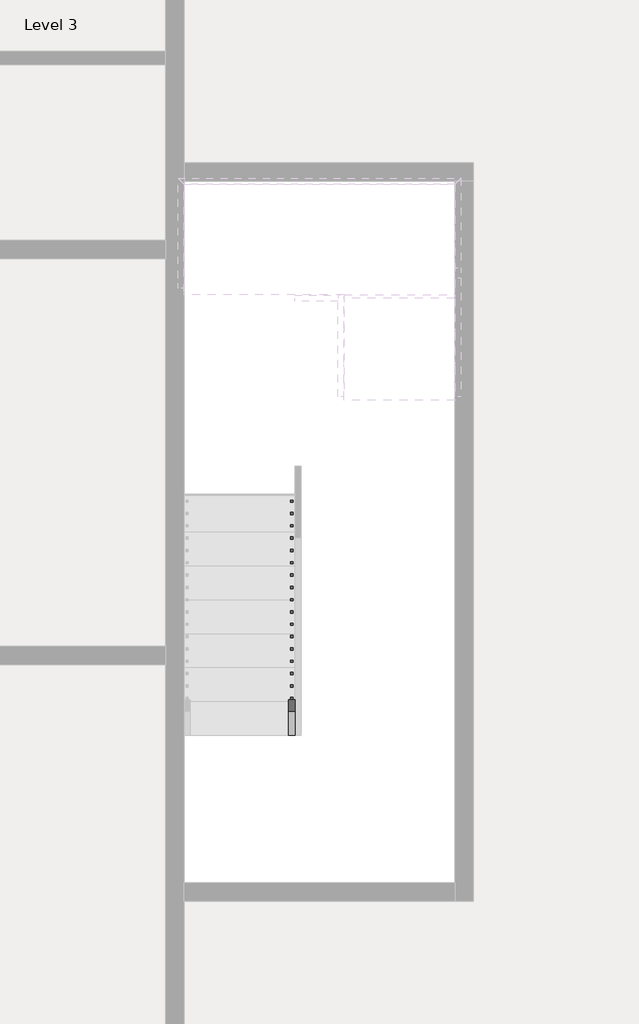
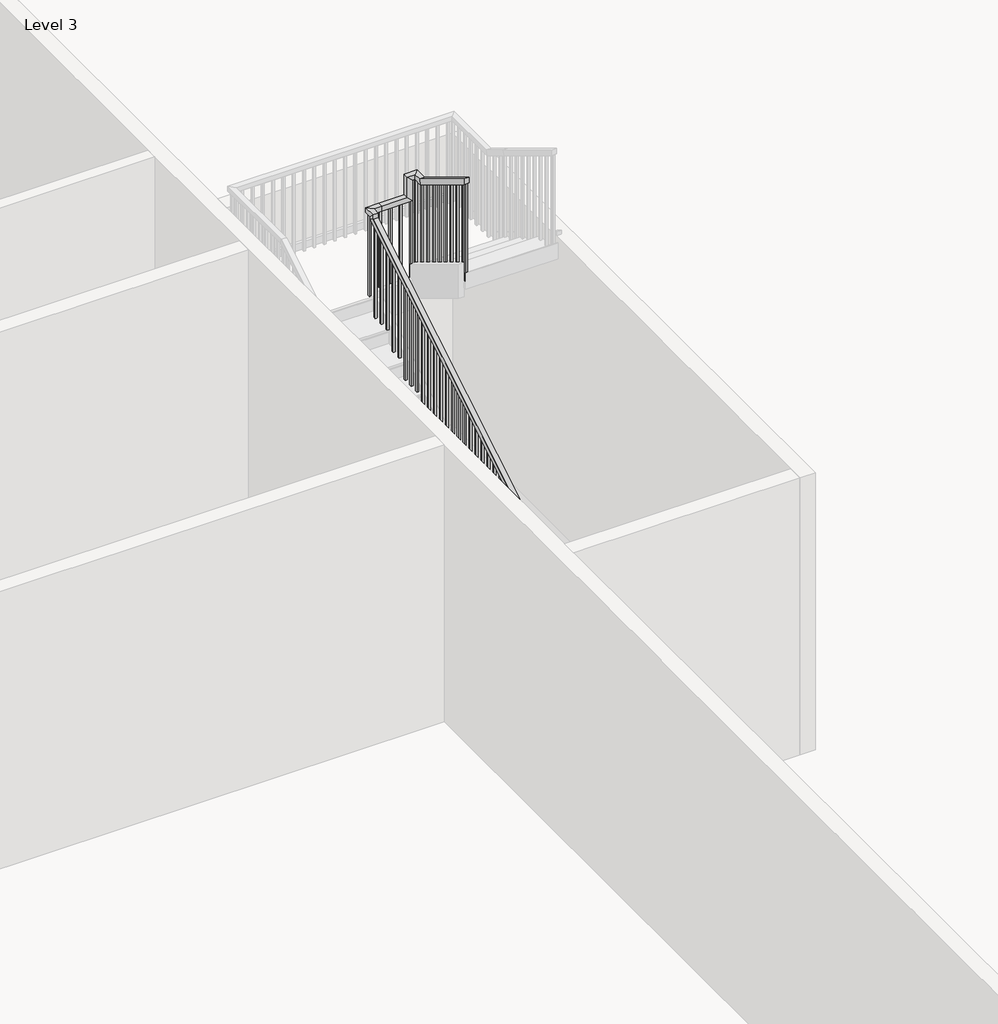
# One storey, part 5 of 8: 1 railing.
"""IFC4 building model written with IfcOpenShell, lengths in millimetres."""

from ifc_helpers import new_model, si_unit, frame, origin, place, context, project, spatial, polyline, outline, extrude, faceted_brep, element, save

model = new_model("IFC4")

# Units and contexts
model_context = context("Model", 3, world=origin())
ifc_project = project(units=[si_unit("LENGTHUNIT", "METRE", prefix="MILLI")], contexts=[model_context])

# Site, building, storey
site = spatial("IfcSite", under=ifc_project)
building = spatial("IfcBuilding", under=site)
storey = spatial("IfcBuildingStorey", under=building, Name="Level 3", Elevation=31330.6172466)

# Railing
placement = place(None, origin())
element("IfcRailing", 1, ObjectType="Handrail - Rectangular", at=placement, inside=storey, context=model_context, shape_type="SolidModel", body=[
    faceted_brep([(-2753.8415084, -23154.3851539, 32414.3505799), (-2753.8415084, -23154.3851539, 32354.9491197), (-2703.0415084, -23154.3851539, 32354.9491197), (-2703.0415084, -23154.3851539, 32414.3505799), (-2753.8415084, -19598.3851539, 34569.5020951), (-2753.8415084, -19547.5851539, 34540.8885136), (-2703.0415084, -19547.5851539, 34540.8885136), (-2703.0415084, -19598.3851539, 34569.5020951), (-2753.8415084, -19598.3851539, 34615.6839133), (-2753.8415084, -19547.5851539, 34564.8839133), (-2703.0415084, -19547.5851539, 34564.8839133), (-2703.0415084, -19598.3851539, 34615.6839133), (-2753.8415084, -19471.3851539, 34615.6839133), (-2753.8415084, -19471.3851539, 34564.8839133), (-2703.0415084, -19522.1851539, 34564.8839133), (-2703.0415084, -19522.1851539, 34615.6839133), (-2626.8415084, -19471.3851539, 34615.6839133), (-2626.8415084, -19471.3851539, 34564.8839133), (-2626.8415084, -19522.1851539, 34564.8839133), (-2626.8415084, -19522.1851539, 34615.6839133), (-2372.8415084, -19471.3851539, 34615.6839133), (-2322.0415084, -19471.3851539, 34564.8839133), (-2322.0415084, -19522.1851539, 34564.8839133), (-2372.8415084, -19522.1851539, 34615.6839133), (-2372.8415084, -19471.3851539, 34831.1990648), (-2322.0415084, -19471.3851539, 34780.3990648), (-2322.0415084, -19522.1851539, 34780.3990648), (-2372.8415084, -19522.1851539, 34831.1990648), (-2245.8415084, -19471.3851539, 34831.1990648), (-2245.8415084, -19471.3851539, 34780.3990648), (-2296.6415084, -19522.1851539, 34780.3990648), (-2296.6415084, -19522.1851539, 34831.1990648), (-2245.8415084, -19598.3851539, 34831.1990648), (-2245.8415084, -19612.5775633, 34780.3990648), (-2296.6415084, -19612.5775633, 34780.3990648), (-2296.6415084, -19598.3851539, 34831.1990648), (-2245.8415084, -20360.3851539, 35293.0172466), (-2296.6415084, -20360.3851539, 35293.0172466), (-2296.6415084, -20360.3851539, 35233.6157863), (-2245.8415084, -20360.3851539, 35233.6157863)], [[[0, 1, 2, 3]], [[1, 0, 4, 5]], [[2, 1, 5, 6]], [[3, 2, 6, 7]], [[0, 3, 7, 4]], [[5, 4, 8, 9]], [[6, 5, 9, 10]], [[7, 6, 10, 11]], [[4, 7, 11, 8]], [[9, 8, 12, 13]], [[10, 9, 13, 14]], [[11, 10, 14, 15]], [[8, 11, 15, 12]], [[13, 12, 16, 17]], [[14, 13, 17, 18]], [[15, 14, 18, 19]], [[12, 15, 19, 16]], [[17, 16, 20, 21]], [[18, 17, 21, 22]], [[19, 18, 22, 23]], [[16, 19, 23, 20]], [[21, 20, 24, 25]], [[22, 21, 25, 26]], [[23, 22, 26, 27]], [[20, 23, 27, 24]], [[25, 24, 28, 29]], [[26, 25, 29, 30]], [[27, 26, 30, 31]], [[24, 27, 31, 28]], [[29, 28, 32, 33]], [[30, 29, 33, 34]], [[31, 30, 34, 35]], [[28, 31, 35, 32]], [[36, 37, 38, 39]], [[33, 32, 36, 39]], [[34, 33, 39, 38]], [[35, 34, 38, 37]], [[32, 35, 37, 36]]]),
    extrude(outline(polyline([(-20319.1101539, 35208.6006348), (-20300.0601539, 35197.0551803), (-20300.0601539, 34209.2839133), (-20319.1101539, 34209.2839133), (-20319.1101539, 35208.6006348)])), frame((-2280.7665084, 0.0, 0.0), z_axis=(1.0, 0.0, 0.0), x_axis=(0.0, 1.0, 0.0)), (0.0, 0.0, 1.0), 19.05),
    extrude(outline(polyline([(-20217.5101539, 35147.0248773), (-20198.4601539, 35135.4794227), (-20198.4601539, 34209.2839133), (-20217.5101539, 34209.2839133), (-20217.5101539, 35147.0248773)])), frame((-2280.7665084, 0.0, 0.0), z_axis=(1.0, 0.0, 0.0), x_axis=(0.0, 1.0, 0.0)), (0.0, 0.0, 1.0), 19.05),
    extrude(outline(polyline([(-20115.9101539, 35085.4491197), (-20096.8601539, 35073.9036651), (-20096.8601539, 34209.2839133), (-20115.9101539, 34209.2839133), (-20115.9101539, 35085.4491197)])), frame((-2280.7665084, 0.0, 0.0), z_axis=(1.0, 0.0, 0.0), x_axis=(0.0, 1.0, 0.0)), (0.0, 0.0, 1.0), 19.05),
    extrude(outline(polyline([(-20014.3101539, 35023.8733621), (-19995.2601539, 35012.3279076), (-19995.2601539, 34039.9505799), (-20014.3101539, 34039.9505799), (-20014.3101539, 35023.8733621)])), frame((-2280.7665084, 0.0, 0.0), z_axis=(1.0, 0.0, 0.0), x_axis=(0.0, 1.0, 0.0)), (0.0, 0.0, 1.0), 19.05),
    extrude(outline(polyline([(-19912.7101539, 34962.2976045), (-19893.6601539, 34950.75215), (-19893.6601539, 34039.9505799), (-19912.7101539, 34039.9505799), (-19912.7101539, 34962.2976045)])), frame((-2280.7665084, 0.0, 0.0), z_axis=(1.0, 0.0, 0.0), x_axis=(0.0, 1.0, 0.0)), (0.0, 0.0, 1.0), 19.05),
    extrude(outline(polyline([(-19811.1101539, 34900.721847), (-19792.0601539, 34889.1763924), (-19792.0601539, 34039.9505799), (-19811.1101539, 34039.9505799), (-19811.1101539, 34900.721847)])), frame((-2280.7665084, 0.0, 0.0), z_axis=(1.0, 0.0, 0.0), x_axis=(0.0, 1.0, 0.0)), (0.0, 0.0, 1.0), 19.05),
    extrude(outline(polyline([(-19709.5101539, 34839.1460894), (-19690.4601539, 34827.6006348), (-19690.4601539, 33870.6172466), (-19709.5101539, 33870.6172466), (-19709.5101539, 34839.1460894)])), frame((-2280.7665084, 0.0, 0.0), z_axis=(1.0, 0.0, 0.0), x_axis=(0.0, 1.0, 0.0)), (0.0, 0.0, 1.0), 19.05),
    extrude(outline(polyline([(-19607.9101539, 34777.5703318), (-19588.8601539, 34766.0248773), (-19588.8601539, 33870.6172466), (-19607.9101539, 33870.6172466), (-19607.9101539, 34777.5703318)])), frame((-2280.7665084, 0.0, 0.0), z_axis=(1.0, 0.0, 0.0), x_axis=(0.0, 1.0, 0.0)), (0.0, 0.0, 1.0), 19.05),
    extrude(outline(polyline([(-2331.5665084, -19506.3101539), (-2331.5665084, -19487.2601539), (-2312.5165084, -19487.2601539), (-2312.5165084, -19506.3101539), (-2331.5665084, -19506.3101539)])), frame((0.0, 0.0, 33701.2839133), z_axis=(0.0, 0.0, 1.0), x_axis=(1.0, 0.0, 0.0)), (0.0, 0.0, 1.0), 1079.1151515),
    extrude(outline(polyline([(-2433.1665084, -19506.3101539), (-2433.1665084, -19487.2601539), (-2414.1165084, -19487.2601539), (-2414.1165084, -19506.3101539), (-2433.1665084, -19506.3101539)])), frame((0.0, 0.0, 33701.2839133), z_axis=(0.0, 0.0, 1.0), x_axis=(1.0, 0.0, 0.0)), (0.0, 0.0, 1.0), 863.6),
    extrude(outline(polyline([(-2534.7665084, -19506.3101539), (-2534.7665084, -19487.2601539), (-2515.7165084, -19487.2601539), (-2515.7165084, -19506.3101539), (-2534.7665084, -19506.3101539)])), frame((0.0, 0.0, 33701.2839133), z_axis=(0.0, 0.0, 1.0), x_axis=(1.0, 0.0, 0.0)), (0.0, 0.0, 1.0), 863.6),
    extrude(outline(polyline([(-2636.3665084, -19506.3101539), (-2636.3665084, -19487.2601539), (-2617.3165084, -19487.2601539), (-2617.3165084, -19506.3101539), (-2636.3665084, -19506.3101539)])), frame((0.0, 0.0, 33701.2839133), z_axis=(0.0, 0.0, 1.0), x_axis=(1.0, 0.0, 0.0)), (0.0, 0.0, 1.0), 863.6),
    extrude(outline(polyline([(-19607.9101539, 34504.3279076), (-19588.8601539, 34515.8733621), (-19588.8601539, 33531.9505799), (-19607.9101539, 33531.9505799), (-19607.9101539, 34504.3279076)])), frame((-2737.9665084, 0.0, 0.0), z_axis=(1.0, 0.0, 0.0), x_axis=(0.0, 1.0, 0.0)), (0.0, 0.0, 1.0), 19.05),
    extrude(outline(polyline([(-19709.5101539, 34442.75215), (-19690.4601539, 34454.2976045), (-19690.4601539, 33531.9505799), (-19709.5101539, 33531.9505799), (-19709.5101539, 34442.75215)])), frame((-2737.9665084, 0.0, 0.0), z_axis=(1.0, 0.0, 0.0), x_axis=(0.0, 1.0, 0.0)), (0.0, 0.0, 1.0), 19.05),
    extrude(outline(polyline([(-19811.1101539, 34381.1763924), (-19792.0601539, 34392.721847), (-19792.0601539, 33531.9505799), (-19811.1101539, 33531.9505799), (-19811.1101539, 34381.1763924)])), frame((-2737.9665084, 0.0, 0.0), z_axis=(1.0, 0.0, 0.0), x_axis=(0.0, 1.0, 0.0)), (0.0, 0.0, 1.0), 19.05),
    extrude(outline(polyline([(-19912.7101539, 34319.6006348), (-19893.6601539, 34331.1460894), (-19893.6601539, 33362.6172466), (-19912.7101539, 33362.6172466), (-19912.7101539, 34319.6006348)])), frame((-2737.9665084, 0.0, 0.0), z_axis=(1.0, 0.0, 0.0), x_axis=(0.0, 1.0, 0.0)), (0.0, 0.0, 1.0), 19.05),
    extrude(outline(polyline([(-20014.3101539, 34258.0248773), (-19995.2601539, 34269.5703318), (-19995.2601539, 33362.6172466), (-20014.3101539, 33362.6172466), (-20014.3101539, 34258.0248773)])), frame((-2737.9665084, 0.0, 0.0), z_axis=(1.0, 0.0, 0.0), x_axis=(0.0, 1.0, 0.0)), (0.0, 0.0, 1.0), 19.05),
    extrude(outline(polyline([(-20115.9101539, 34196.4491197), (-20096.8601539, 34207.9945742), (-20096.8601539, 33193.2839133), (-20115.9101539, 33193.2839133), (-20115.9101539, 34196.4491197)])), frame((-2737.9665084, 0.0, 0.0), z_axis=(1.0, 0.0, 0.0), x_axis=(0.0, 1.0, 0.0)), (0.0, 0.0, 1.0), 19.05),
    extrude(outline(polyline([(-20217.5101539, 34134.8733621), (-20198.4601539, 34146.4188166), (-20198.4601539, 33193.2839133), (-20217.5101539, 33193.2839133), (-20217.5101539, 34134.8733621)])), frame((-2737.9665084, 0.0, 0.0), z_axis=(1.0, 0.0, 0.0), x_axis=(0.0, 1.0, 0.0)), (0.0, 0.0, 1.0), 19.05),
    extrude(outline(polyline([(-20319.1101539, 34073.2976045), (-20300.0601539, 34084.8430591), (-20300.0601539, 33193.2839133), (-20319.1101539, 33193.2839133), (-20319.1101539, 34073.2976045)])), frame((-2737.9665084, 0.0, 0.0), z_axis=(1.0, 0.0, 0.0), x_axis=(0.0, 1.0, 0.0)), (0.0, 0.0, 1.0), 19.05),
    extrude(outline(polyline([(-20420.7101539, 34011.721847), (-20401.6601539, 34023.2673015), (-20401.6601539, 33023.9505799), (-20420.7101539, 33023.9505799), (-20420.7101539, 34011.721847)])), frame((-2737.9665084, 0.0, 0.0), z_axis=(1.0, 0.0, 0.0), x_axis=(0.0, 1.0, 0.0)), (0.0, 0.0, 1.0), 19.05),
    extrude(outline(polyline([(-20522.3101539, 33950.1460894), (-20503.2601539, 33961.6915439), (-20503.2601539, 33023.9505799), (-20522.3101539, 33023.9505799), (-20522.3101539, 33950.1460894)])), frame((-2737.9665084, 0.0, 0.0), z_axis=(1.0, 0.0, 0.0), x_axis=(0.0, 1.0, 0.0)), (0.0, 0.0, 1.0), 19.05),
    extrude(outline(polyline([(-20623.9101539, 33888.5703318), (-20604.8601539, 33900.1157863), (-20604.8601539, 33023.9505799), (-20623.9101539, 33023.9505799), (-20623.9101539, 33888.5703318)])), frame((-2737.9665084, 0.0, 0.0), z_axis=(1.0, 0.0, 0.0), x_axis=(0.0, 1.0, 0.0)), (0.0, 0.0, 1.0), 19.05),
    extrude(outline(polyline([(-20725.5101539, 33826.9945742), (-20706.4601539, 33838.5400288), (-20706.4601539, 32854.6172466), (-20725.5101539, 32854.6172466), (-20725.5101539, 33826.9945742)])), frame((-2737.9665084, 0.0, 0.0), z_axis=(1.0, 0.0, 0.0), x_axis=(0.0, 1.0, 0.0)), (0.0, 0.0, 1.0), 19.05),
    extrude(outline(polyline([(-20827.1101539, 33765.4188166), (-20808.0601539, 33776.9642712), (-20808.0601539, 32854.6172466), (-20827.1101539, 32854.6172466), (-20827.1101539, 33765.4188166)])), frame((-2737.9665084, 0.0, 0.0), z_axis=(1.0, 0.0, 0.0), x_axis=(0.0, 1.0, 0.0)), (0.0, 0.0, 1.0), 19.05),
    extrude(outline(polyline([(-20928.7101539, 33703.8430591), (-20909.6601539, 33715.3885136), (-20909.6601539, 32854.6172466), (-20928.7101539, 32854.6172466), (-20928.7101539, 33703.8430591)])), frame((-2737.9665084, 0.0, 0.0), z_axis=(1.0, 0.0, 0.0), x_axis=(0.0, 1.0, 0.0)), (0.0, 0.0, 1.0), 19.05),
    extrude(outline(polyline([(-21030.3101539, 33642.2673015), (-21011.2601539, 33653.812756), (-21011.2601539, 32685.2839133), (-21030.3101539, 32685.2839133), (-21030.3101539, 33642.2673015)])), frame((-2737.9665084, 0.0, 0.0), z_axis=(1.0, 0.0, 0.0), x_axis=(0.0, 1.0, 0.0)), (0.0, 0.0, 1.0), 19.05),
    extrude(outline(polyline([(-21131.9101539, 33580.6915439), (-21112.8601539, 33592.2369985), (-21112.8601539, 32685.2839133), (-21131.9101539, 32685.2839133), (-21131.9101539, 33580.6915439)])), frame((-2737.9665084, 0.0, 0.0), z_axis=(1.0, 0.0, 0.0), x_axis=(0.0, 1.0, 0.0)), (0.0, 0.0, 1.0), 19.05),
    extrude(outline(polyline([(-21233.5101539, 33519.1157863), (-21214.4601539, 33530.6612409), (-21214.4601539, 32515.9505799), (-21233.5101539, 32515.9505799), (-21233.5101539, 33519.1157863)])), frame((-2737.9665084, 0.0, 0.0), z_axis=(1.0, 0.0, 0.0), x_axis=(0.0, 1.0, 0.0)), (0.0, 0.0, 1.0), 19.05),
    extrude(outline(polyline([(-21335.1101539, 33457.5400288), (-21316.0601539, 33469.0854833), (-21316.0601539, 32515.9505799), (-21335.1101539, 32515.9505799), (-21335.1101539, 33457.5400288)])), frame((-2737.9665084, 0.0, 0.0), z_axis=(1.0, 0.0, 0.0), x_axis=(0.0, 1.0, 0.0)), (0.0, 0.0, 1.0), 19.05),
    extrude(outline(polyline([(-21436.7101539, 33395.9642712), (-21417.6601539, 33407.5097257), (-21417.6601539, 32515.9505799), (-21436.7101539, 32515.9505799), (-21436.7101539, 33395.9642712)])), frame((-2737.9665084, 0.0, 0.0), z_axis=(1.0, 0.0, 0.0), x_axis=(0.0, 1.0, 0.0)), (0.0, 0.0, 1.0), 19.05),
    extrude(outline(polyline([(-21538.3101539, 33334.3885136), (-21519.2601539, 33345.9339682), (-21519.2601539, 32346.6172466), (-21538.3101539, 32346.6172466), (-21538.3101539, 33334.3885136)])), frame((-2737.9665084, 0.0, 0.0), z_axis=(1.0, 0.0, 0.0), x_axis=(0.0, 1.0, 0.0)), (0.0, 0.0, 1.0), 19.05),
    extrude(outline(polyline([(-21639.9101539, 33272.812756), (-21620.8601539, 33284.3582106), (-21620.8601539, 32346.6172466), (-21639.9101539, 32346.6172466), (-21639.9101539, 33272.812756)])), frame((-2737.9665084, 0.0, 0.0), z_axis=(1.0, 0.0, 0.0), x_axis=(0.0, 1.0, 0.0)), (0.0, 0.0, 1.0), 19.05),
    extrude(outline(polyline([(-21741.5101539, 33211.2369985), (-21722.4601539, 33222.782453), (-21722.4601539, 32346.6172466), (-21741.5101539, 32346.6172466), (-21741.5101539, 33211.2369985)])), frame((-2737.9665084, 0.0, 0.0), z_axis=(1.0, 0.0, 0.0), x_axis=(0.0, 1.0, 0.0)), (0.0, 0.0, 1.0), 19.05),
    extrude(outline(polyline([(-21843.1101539, 33149.6612409), (-21824.0601539, 33161.2066954), (-21824.0601539, 32177.2839133), (-21843.1101539, 32177.2839133), (-21843.1101539, 33149.6612409)])), frame((-2737.9665084, 0.0, 0.0), z_axis=(1.0, 0.0, 0.0), x_axis=(0.0, 1.0, 0.0)), (0.0, 0.0, 1.0), 19.05),
    extrude(outline(polyline([(-21944.7101539, 33088.0854833), (-21925.6601539, 33099.6309379), (-21925.6601539, 32177.2839133), (-21944.7101539, 32177.2839133), (-21944.7101539, 33088.0854833)])), frame((-2737.9665084, 0.0, 0.0), z_axis=(1.0, 0.0, 0.0), x_axis=(0.0, 1.0, 0.0)), (0.0, 0.0, 1.0), 19.05),
    extrude(outline(polyline([(-22046.3101539, 33026.5097257), (-22027.2601539, 33038.0551803), (-22027.2601539, 32177.2839133), (-22046.3101539, 32177.2839133), (-22046.3101539, 33026.5097257)])), frame((-2737.9665084, 0.0, 0.0), z_axis=(1.0, 0.0, 0.0), x_axis=(0.0, 1.0, 0.0)), (0.0, 0.0, 1.0), 19.05),
    extrude(outline(polyline([(-22147.9101539, 32964.9339682), (-22128.8601539, 32976.4794227), (-22128.8601539, 32007.9505799), (-22147.9101539, 32007.9505799), (-22147.9101539, 32964.9339682)])), frame((-2737.9665084, 0.0, 0.0), z_axis=(1.0, 0.0, 0.0), x_axis=(0.0, 1.0, 0.0)), (0.0, 0.0, 1.0), 19.05),
    extrude(outline(polyline([(-22249.5101539, 32903.3582106), (-22230.4601539, 32914.9036651), (-22230.4601539, 32007.9505799), (-22249.5101539, 32007.9505799), (-22249.5101539, 32903.3582106)])), frame((-2737.9665084, 0.0, 0.0), z_axis=(1.0, 0.0, 0.0), x_axis=(0.0, 1.0, 0.0)), (0.0, 0.0, 1.0), 19.05),
    extrude(outline(polyline([(-22351.1101539, 32841.782453), (-22332.0601539, 32853.3279076), (-22332.0601539, 31838.6172466), (-22351.1101539, 31838.6172466), (-22351.1101539, 32841.782453)])), frame((-2737.9665084, 0.0, 0.0), z_axis=(1.0, 0.0, 0.0), x_axis=(0.0, 1.0, 0.0)), (0.0, 0.0, 1.0), 19.05),
    extrude(outline(polyline([(-22452.7101539, 32780.2066954), (-22433.6601539, 32791.75215), (-22433.6601539, 31838.6172466), (-22452.7101539, 31838.6172466), (-22452.7101539, 32780.2066954)])), frame((-2737.9665084, 0.0, 0.0), z_axis=(1.0, 0.0, 0.0), x_axis=(0.0, 1.0, 0.0)), (0.0, 0.0, 1.0), 19.05),
    extrude(outline(polyline([(-22554.3101539, 32718.6309379), (-22535.2601539, 32730.1763924), (-22535.2601539, 31838.6172466), (-22554.3101539, 31838.6172466), (-22554.3101539, 32718.6309379)])), frame((-2737.9665084, 0.0, 0.0), z_axis=(1.0, 0.0, 0.0), x_axis=(0.0, 1.0, 0.0)), (0.0, 0.0, 1.0), 19.05),
    extrude(outline(polyline([(-22655.9101539, 32657.0551803), (-22636.8601539, 32668.6006348), (-22636.8601539, 31669.2839133), (-22655.9101539, 31669.2839133), (-22655.9101539, 32657.0551803)])), frame((-2737.9665084, 0.0, 0.0), z_axis=(1.0, 0.0, 0.0), x_axis=(0.0, 1.0, 0.0)), (0.0, 0.0, 1.0), 19.05),
    extrude(outline(polyline([(-22757.5101539, 32595.4794227), (-22738.4601539, 32607.0248773), (-22738.4601539, 31669.2839133), (-22757.5101539, 31669.2839133), (-22757.5101539, 32595.4794227)])), frame((-2737.9665084, 0.0, 0.0), z_axis=(1.0, 0.0, 0.0), x_axis=(0.0, 1.0, 0.0)), (0.0, 0.0, 1.0), 19.05),
    extrude(outline(polyline([(-22859.1101539, 32533.9036651), (-22840.0601539, 32545.4491197), (-22840.0601539, 31669.2839133), (-22859.1101539, 31669.2839133), (-22859.1101539, 32533.9036651)])), frame((-2737.9665084, 0.0, 0.0), z_axis=(1.0, 0.0, 0.0), x_axis=(0.0, 1.0, 0.0)), (0.0, 0.0, 1.0), 19.05),
    extrude(outline(polyline([(-22960.7101539, 32472.3279076), (-22941.6601539, 32483.8733621), (-22941.6601539, 31499.9505799), (-22960.7101539, 31499.9505799), (-22960.7101539, 32472.3279076)])), frame((-2737.9665084, 0.0, 0.0), z_axis=(1.0, 0.0, 0.0), x_axis=(0.0, 1.0, 0.0)), (0.0, 0.0, 1.0), 19.05),
    extrude(outline(polyline([(-23062.3101539, 32410.75215), (-23043.2601539, 32422.2976045), (-23043.2601539, 31499.9505799), (-23062.3101539, 31499.9505799), (-23062.3101539, 32410.75215)])), frame((-2737.9665084, 0.0, 0.0), z_axis=(1.0, 0.0, 0.0), x_axis=(0.0, 1.0, 0.0)), (0.0, 0.0, 1.0), 19.05),
    extrude(outline(polyline([(-2280.7665084, -19506.3101539), (-2280.7665084, -19487.2601539), (-2261.7165084, -19487.2601539), (-2261.7165084, -19506.3101539), (-2280.7665084, -19506.3101539)])), frame((0.0, 0.0, 33701.2839133), z_axis=(0.0, 0.0, 1.0), x_axis=(1.0, 0.0, 0.0)), (0.0, 0.0, 1.0), 1079.1151515),
    extrude(outline(polyline([(-2718.9165084, -19506.3101539), (-2737.9665084, -19506.3101539), (-2737.9665084, -19487.2601539), (-2718.9165084, -19487.2601539), (-2718.9165084, -19506.3101539)])), frame((0.0, 0.0, 33701.2839133), z_axis=(0.0, 0.0, 1.0), x_axis=(1.0, 0.0, 0.0)), (0.0, 0.0, 1.0), 863.6),
    extrude(outline(polyline([(-20360.3851539, 35233.6157863), (-20341.3351539, 35222.0703318), (-20341.3351539, 34209.2839133), (-20360.3851539, 34209.2839133), (-20360.3851539, 35233.6157863)])), frame((-2280.7665084, 0.0, 0.0), z_axis=(1.0, 0.0, 0.0), x_axis=(0.0, 1.0, 0.0)), (0.0, 0.0, 1.0), 19.05),
    extrude(outline(polyline([(-23154.3851539, 32354.9491197), (-23135.3351539, 32366.4945742), (-23135.3351539, 31499.9505799), (-23154.3851539, 31499.9505799), (-23154.3851539, 32354.9491197)])), frame((-2737.9665084, 0.0, 0.0), z_axis=(1.0, 0.0, 0.0), x_axis=(0.0, 1.0, 0.0)), (0.0, 0.0, 1.0), 19.05),
])

save(model, "model.ifc")

# Revit data of these elements
# Type "Handrail - Rectangular"
#   Assembly Code = "C2010400"
#   built-in parameter 1008612 = 0.0416667 (stored number, unit not read)
#   built-in parameter 1008611 = 0.0416667 (stored number, unit not read)
#   built-in parameter 1008609 = 0.333333 (stored number, unit not read)
#   built-in parameter 1008604 = 0.166667 (stored number, unit not read)
#   built-in parameter 1008603 = 0.166667 (stored number, unit not read)
#   Railing Height = 3' - 0"
#   built-in parameter 1008630 = 2
#   built-in parameter 1008610 = 2
#   built-in parameter 1008618 = Baluster - Square : 3/4"
# Element 1 (IfcRailing, "Handrail - Rectangular")
#   Phase Created = New Construction
